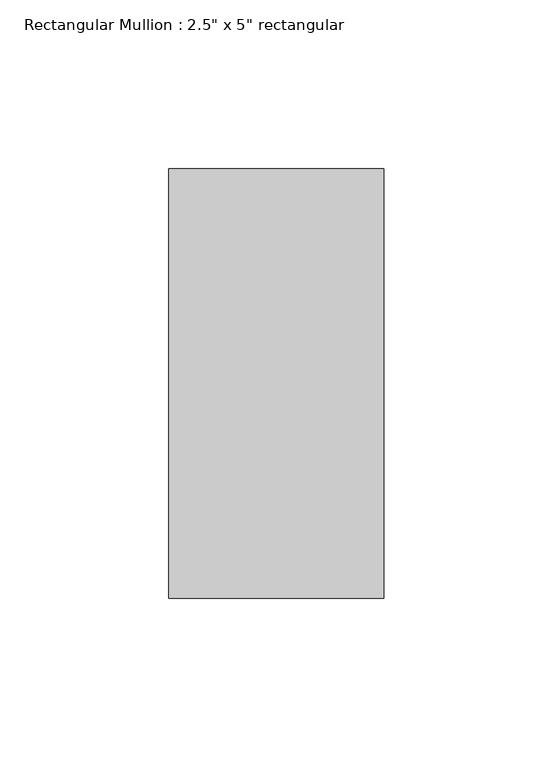
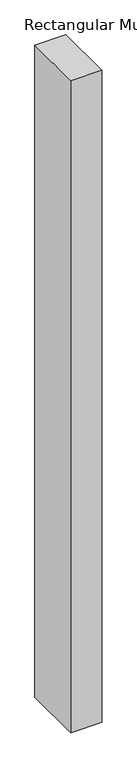
"""IFC4 building model written with IfcOpenShell, lengths in millimetres: member geometry."""

from ifc_helpers import new_model, si_unit, frame, origin, place, context, project, spatial, polyline, outline, extrude, source, transform, mapped, element, save


def member_12fb2005(model_context):
    return source(origin(), model_context, "Body", "SweptSolid", [
        extrude(outline(polyline([(0.0, 63.5), (0.0, -63.5), (-63.5, -63.5), (-63.5, 63.5), (0.0, 63.5)])), frame((0.0, 0.0, -1411.7908292), z_axis=(0.0, 0.0, 1.0), x_axis=(1.0, 0.0, 0.0)), (0.0, 0.0, 1.0), 1411.7908292),
    ])


if __name__ == "__main__":
    model = new_model("IFC4")
    model_context = context("Model", 3, world=origin())
    ifc_project = project(units=[si_unit("LENGTHUNIT", "METRE", prefix="MILLI")], contexts=[model_context])
    site = spatial("IfcSite", under=ifc_project)
    building = spatial("IfcBuilding", under=site)
    placement = place(None, origin())
    member_shape = member_12fb2005(model_context)
    element("IfcMember", 1, ObjectType="Rectangular Mullion : 2.5\" x 5\" rectangular", at=placement, inside=building, context=model_context, shape_type="MappedRepresentation", body=[
        mapped(member_shape, transform((0.0, 0.0, 0.0), x_axis=(1.0, 0.0, 0.0), y_axis=(0.0, 1.0, 0.0), z_axis=(0.0, 0.0, 1.0))),
    ])
    save(model, "model.ifc")

# Revit data of these elements
# Type "Rectangular Mullion : 2.5\" x 5\" rectangular"
#   built-in parameter 1007304 = 0.416667 (stored number, unit not read)
#   built-in parameter 1007301 = 0.104167 (stored number, unit not read)
#   built-in parameter 1007300 = 0.104167 (stored number, unit not read)
# Element 1 (IfcMember, "Rectangular Mullion : 2.5\" x 5\" rectangular")
#   Materials on its faces: "Aluminum"
# Materials
#   "Aluminum": class "Metal", colour RGB 247 247 247, transparency 0, Description = "Aluminum 6061", Cost = 0
